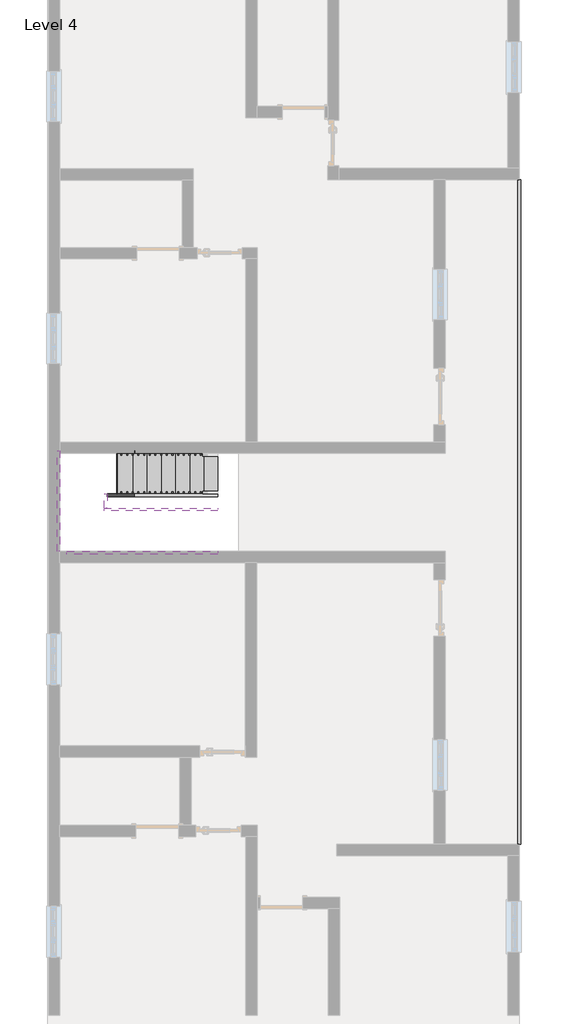
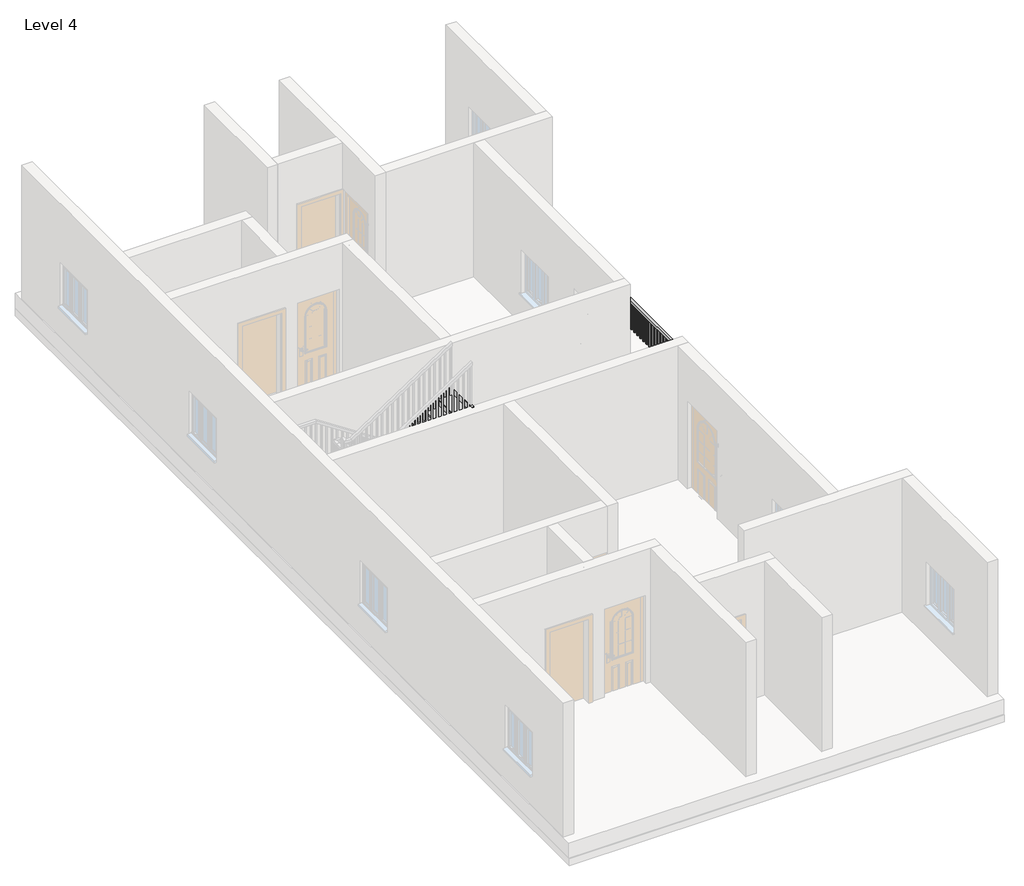
# One storey, part 3 of 3: 6 members, 1 railing, 1 stair flight.
"""IFC4 building model written with IfcOpenShell, lengths in millimetres."""

from ifc_helpers import new_model, si_unit, frame, origin, place, context, project, spatial, polyline, outline, extrude, transform, mapped, element, save
from components import stair_flight_94c6aef5

model = new_model("IFC4")

# Units and contexts
model_context = context("Model", 3, world=origin())
ifc_project = project(units=[si_unit("LENGTHUNIT", "METRE", prefix="MILLI")], contexts=[model_context])

# Site, building, storey
site = spatial("IfcSite", under=ifc_project)
building = spatial("IfcBuilding", under=site)
storey = spatial("IfcBuildingStorey", under=building, Name="Level 4", Elevation=9144.0)

# Members
placement = place(None, origin())
element("IfcMember", 1, ObjectType="Stringer - 2\" Width", at=placement, inside=storey, context=model_context, shape_type="SweptSolid", body=[
    extrude(outline(polyline([(9144.0, -2118.1728655), (9361.4747739, -2118.1728655), (10671.2681072, -4099.3728655), (10305.8806735, -4099.3728655), (9144.0, -2341.9063005), (9144.0, -2118.1728655)])), frame((0.0, 417.8797121, 0.0), z_axis=(0.0, 1.0, 0.0), x_axis=(0.0, 0.0, 1.0)), (0.0, 0.0, 1.0), 50.8),
])
element("IfcMember", 2, ObjectType="Stringer - 2\" Width", at=placement, inside=storey, context=model_context, shape_type="SweptSolid", body=[
    extrude(outline(polyline([(-4150.1728655, 468.6797121), (-4099.3728655, 468.6797121), (-4099.3728655, 214.6797121), (-4150.1728655, 214.6797121), (-4150.1728655, 468.6797121)])), frame((0.0, 0.0, 10426.7), z_axis=(0.0, 0.0, 1.0), x_axis=(1.0, 0.0, 0.0)), (0.0, 0.0, 1.0), 304.8),
])
element("IfcMember", 3, ObjectType="Stringer - 2\" Width", at=placement, inside=storey, context=model_context, shape_type="SweptSolid", body=[
    extrude(outline(polyline([(10872.7747739, -4150.1728655), (10507.3873402, -4150.1728655), (11850.765118, -2118.1728655), (12216.1525517, -2118.1728655), (10872.7747739, -4150.1728655)])), frame((0.0, 163.8797121, 0.0), z_axis=(0.0, 1.0, 0.0), x_axis=(0.0, 0.0, 1.0)), (0.0, 0.0, 1.0), 50.8),
])
element("IfcMember", 4, ObjectType="Stringer - 2\" Width", at=placement, inside=storey, context=model_context, shape_type="SweptSolid", body=[
    extrude(outline(polyline([(9144.0, -2118.1728655), (9361.4747739, -2118.1728655), (10731.5, -4190.4799301), (10731.5, -4743.1668047), (9144.0, -2341.9063005), (9144.0, -2118.1728655)])), frame((0.0, 1192.5797121, 0.0), z_axis=(0.0, 1.0, 0.0), x_axis=(0.0, 0.0, 1.0)), (0.0, 0.0, 1.0), 50.8),
])
element("IfcMember", 5, ObjectType="Stringer - 2\" Width", at=placement, inside=storey, context=model_context, shape_type="SweptSolid", body=[
    extrude(outline(polyline([(-4994.7394105, 1243.3797121), (-4943.9394105, 1243.3797121), (-4943.9394105, -560.0202879), (-4994.7394105, -560.0202879), (-4994.7394105, 1243.3797121)])), frame((0.0, 0.0, 10426.7), z_axis=(0.0, 0.0, 1.0), x_axis=(1.0, 0.0, 0.0)), (0.0, 0.0, 1.0), 304.8),
])
element("IfcMember", 6, ObjectType="Stringer - 2\" Width", at=placement, inside=storey, context=model_context, shape_type="SweptSolid", body=[
    extrude(outline(polyline([(10426.7, -4272.2209431), (11850.765118, -2118.1728655), (12216.1525517, -2118.1728655), (10426.7, -4824.9078176), (10426.7, -4272.2209431)])), frame((0.0, -610.8202879, 0.0), z_axis=(0.0, 1.0, 0.0), x_axis=(0.0, 0.0, 1.0)), (0.0, 0.0, 1.0), 50.8),
])

# Railing
element("IfcRailing", 7, ObjectType="Handrail - Rectangular", at=placement, inside=storey, context=model_context, shape_type="SweptSolid", body=[
    extrude(outline(polyline([(3298.3605895, -5805.1202879), (3247.5605895, -5805.1202879), (3247.5605895, 6094.2483916), (3298.3605895, 6094.2483916), (3298.3605895, -5805.1202879)])), frame((0.0, 0.0, 10007.6), z_axis=(0.0, 0.0, 1.0), x_axis=(1.0, 0.0, 0.0)), (0.0, 0.0, 1.0), 50.8),
    extrude(outline(polyline([(3282.4855895, 6072.5547121), (3263.4355895, 6072.5547121), (3263.4355895, 6091.6047121), (3282.4855895, 6091.6047121), (3282.4855895, 6072.5547121)])), frame((0.0, 0.0, 9144.0), z_axis=(0.0, 0.0, 1.0), x_axis=(1.0, 0.0, 0.0)), (0.0, 0.0, 1.0), 863.6),
    extrude(outline(polyline([(3282.4855895, 5970.9547121), (3263.4355895, 5970.9547121), (3263.4355895, 5990.0047121), (3282.4855895, 5990.0047121), (3282.4855895, 5970.9547121)])), frame((0.0, 0.0, 9144.0), z_axis=(0.0, 0.0, 1.0), x_axis=(1.0, 0.0, 0.0)), (0.0, 0.0, 1.0), 863.6),
    extrude(outline(polyline([(3282.4855895, 5869.3547121), (3263.4355895, 5869.3547121), (3263.4355895, 5888.4047121), (3282.4855895, 5888.4047121), (3282.4855895, 5869.3547121)])), frame((0.0, 0.0, 9144.0), z_axis=(0.0, 0.0, 1.0), x_axis=(1.0, 0.0, 0.0)), (0.0, 0.0, 1.0), 863.6),
    extrude(outline(polyline([(3282.4855895, 5767.7547121), (3263.4355895, 5767.7547121), (3263.4355895, 5786.8047121), (3282.4855895, 5786.8047121), (3282.4855895, 5767.7547121)])), frame((0.0, 0.0, 9144.0), z_axis=(0.0, 0.0, 1.0), x_axis=(1.0, 0.0, 0.0)), (0.0, 0.0, 1.0), 863.6),
    extrude(outline(polyline([(3282.4855895, 5666.1547121), (3263.4355895, 5666.1547121), (3263.4355895, 5685.2047121), (3282.4855895, 5685.2047121), (3282.4855895, 5666.1547121)])), frame((0.0, 0.0, 9144.0), z_axis=(0.0, 0.0, 1.0), x_axis=(1.0, 0.0, 0.0)), (0.0, 0.0, 1.0), 863.6),
    extrude(outline(polyline([(3282.4855895, 5564.5547121), (3263.4355895, 5564.5547121), (3263.4355895, 5583.6047121), (3282.4855895, 5583.6047121), (3282.4855895, 5564.5547121)])), frame((0.0, 0.0, 9144.0), z_axis=(0.0, 0.0, 1.0), x_axis=(1.0, 0.0, 0.0)), (0.0, 0.0, 1.0), 863.6),
    extrude(outline(polyline([(3282.4855895, 5462.9547121), (3263.4355895, 5462.9547121), (3263.4355895, 5482.0047121), (3282.4855895, 5482.0047121), (3282.4855895, 5462.9547121)])), frame((0.0, 0.0, 9144.0), z_axis=(0.0, 0.0, 1.0), x_axis=(1.0, 0.0, 0.0)), (0.0, 0.0, 1.0), 863.6),
    extrude(outline(polyline([(3282.4855895, 5361.3547121), (3263.4355895, 5361.3547121), (3263.4355895, 5380.4047121), (3282.4855895, 5380.4047121), (3282.4855895, 5361.3547121)])), frame((0.0, 0.0, 9144.0), z_axis=(0.0, 0.0, 1.0), x_axis=(1.0, 0.0, 0.0)), (0.0, 0.0, 1.0), 863.6),
    extrude(outline(polyline([(3282.4855895, 5259.7547121), (3263.4355895, 5259.7547121), (3263.4355895, 5278.8047121), (3282.4855895, 5278.8047121), (3282.4855895, 5259.7547121)])), frame((0.0, 0.0, 9144.0), z_axis=(0.0, 0.0, 1.0), x_axis=(1.0, 0.0, 0.0)), (0.0, 0.0, 1.0), 863.6),
    extrude(outline(polyline([(3282.4855895, 5158.1547121), (3263.4355895, 5158.1547121), (3263.4355895, 5177.2047121), (3282.4855895, 5177.2047121), (3282.4855895, 5158.1547121)])), frame((0.0, 0.0, 9144.0), z_axis=(0.0, 0.0, 1.0), x_axis=(1.0, 0.0, 0.0)), (0.0, 0.0, 1.0), 863.6),
    extrude(outline(polyline([(3282.4855895, 5056.5547121), (3263.4355895, 5056.5547121), (3263.4355895, 5075.6047121), (3282.4855895, 5075.6047121), (3282.4855895, 5056.5547121)])), frame((0.0, 0.0, 9144.0), z_axis=(0.0, 0.0, 1.0), x_axis=(1.0, 0.0, 0.0)), (0.0, 0.0, 1.0), 863.6),
    extrude(outline(polyline([(3282.4855895, 4954.9547121), (3263.4355895, 4954.9547121), (3263.4355895, 4974.0047121), (3282.4855895, 4974.0047121), (3282.4855895, 4954.9547121)])), frame((0.0, 0.0, 9144.0), z_axis=(0.0, 0.0, 1.0), x_axis=(1.0, 0.0, 0.0)), (0.0, 0.0, 1.0), 863.6),
    extrude(outline(polyline([(3282.4855895, 4853.3547121), (3263.4355895, 4853.3547121), (3263.4355895, 4872.4047121), (3282.4855895, 4872.4047121), (3282.4855895, 4853.3547121)])), frame((0.0, 0.0, 9144.0), z_axis=(0.0, 0.0, 1.0), x_axis=(1.0, 0.0, 0.0)), (0.0, 0.0, 1.0), 863.6),
    extrude(outline(polyline([(3282.4855895, 4751.7547121), (3263.4355895, 4751.7547121), (3263.4355895, 4770.8047121), (3282.4855895, 4770.8047121), (3282.4855895, 4751.7547121)])), frame((0.0, 0.0, 9144.0), z_axis=(0.0, 0.0, 1.0), x_axis=(1.0, 0.0, 0.0)), (0.0, 0.0, 1.0), 863.6),
    extrude(outline(polyline([(3282.4855895, 4650.1547121), (3263.4355895, 4650.1547121), (3263.4355895, 4669.2047121), (3282.4855895, 4669.2047121), (3282.4855895, 4650.1547121)])), frame((0.0, 0.0, 9144.0), z_axis=(0.0, 0.0, 1.0), x_axis=(1.0, 0.0, 0.0)), (0.0, 0.0, 1.0), 863.6),
    extrude(outline(polyline([(3282.4855895, 4548.5547121), (3263.4355895, 4548.5547121), (3263.4355895, 4567.6047121), (3282.4855895, 4567.6047121), (3282.4855895, 4548.5547121)])), frame((0.0, 0.0, 9144.0), z_axis=(0.0, 0.0, 1.0), x_axis=(1.0, 0.0, 0.0)), (0.0, 0.0, 1.0), 863.6),
    extrude(outline(polyline([(3282.4855895, 4446.9547121), (3263.4355895, 4446.9547121), (3263.4355895, 4466.0047121), (3282.4855895, 4466.0047121), (3282.4855895, 4446.9547121)])), frame((0.0, 0.0, 9144.0), z_axis=(0.0, 0.0, 1.0), x_axis=(1.0, 0.0, 0.0)), (0.0, 0.0, 1.0), 863.6),
    extrude(outline(polyline([(3282.4855895, 4345.3547121), (3263.4355895, 4345.3547121), (3263.4355895, 4364.4047121), (3282.4855895, 4364.4047121), (3282.4855895, 4345.3547121)])), frame((0.0, 0.0, 9144.0), z_axis=(0.0, 0.0, 1.0), x_axis=(1.0, 0.0, 0.0)), (0.0, 0.0, 1.0), 863.6),
    extrude(outline(polyline([(3282.4855895, 4243.7547121), (3263.4355895, 4243.7547121), (3263.4355895, 4262.8047121), (3282.4855895, 4262.8047121), (3282.4855895, 4243.7547121)])), frame((0.0, 0.0, 9144.0), z_axis=(0.0, 0.0, 1.0), x_axis=(1.0, 0.0, 0.0)), (0.0, 0.0, 1.0), 863.6),
    extrude(outline(polyline([(3282.4855895, 4142.1547121), (3263.4355895, 4142.1547121), (3263.4355895, 4161.2047121), (3282.4855895, 4161.2047121), (3282.4855895, 4142.1547121)])), frame((0.0, 0.0, 9144.0), z_axis=(0.0, 0.0, 1.0), x_axis=(1.0, 0.0, 0.0)), (0.0, 0.0, 1.0), 863.6),
    extrude(outline(polyline([(3282.4855895, 4040.5547121), (3263.4355895, 4040.5547121), (3263.4355895, 4059.6047121), (3282.4855895, 4059.6047121), (3282.4855895, 4040.5547121)])), frame((0.0, 0.0, 9144.0), z_axis=(0.0, 0.0, 1.0), x_axis=(1.0, 0.0, 0.0)), (0.0, 0.0, 1.0), 863.6),
    extrude(outline(polyline([(3282.4855895, 3938.9547121), (3263.4355895, 3938.9547121), (3263.4355895, 3958.0047121), (3282.4855895, 3958.0047121), (3282.4855895, 3938.9547121)])), frame((0.0, 0.0, 9144.0), z_axis=(0.0, 0.0, 1.0), x_axis=(1.0, 0.0, 0.0)), (0.0, 0.0, 1.0), 863.6),
    extrude(outline(polyline([(3282.4855895, 3837.3547121), (3263.4355895, 3837.3547121), (3263.4355895, 3856.4047121), (3282.4855895, 3856.4047121), (3282.4855895, 3837.3547121)])), frame((0.0, 0.0, 9144.0), z_axis=(0.0, 0.0, 1.0), x_axis=(1.0, 0.0, 0.0)), (0.0, 0.0, 1.0), 863.6),
    extrude(outline(polyline([(3282.4855895, 3735.7547121), (3263.4355895, 3735.7547121), (3263.4355895, 3754.8047121), (3282.4855895, 3754.8047121), (3282.4855895, 3735.7547121)])), frame((0.0, 0.0, 9144.0), z_axis=(0.0, 0.0, 1.0), x_axis=(1.0, 0.0, 0.0)), (0.0, 0.0, 1.0), 863.6),
    extrude(outline(polyline([(3282.4855895, 3634.1547121), (3263.4355895, 3634.1547121), (3263.4355895, 3653.2047121), (3282.4855895, 3653.2047121), (3282.4855895, 3634.1547121)])), frame((0.0, 0.0, 9144.0), z_axis=(0.0, 0.0, 1.0), x_axis=(1.0, 0.0, 0.0)), (0.0, 0.0, 1.0), 863.6),
    extrude(outline(polyline([(3282.4855895, 3532.5547121), (3263.4355895, 3532.5547121), (3263.4355895, 3551.6047121), (3282.4855895, 3551.6047121), (3282.4855895, 3532.5547121)])), frame((0.0, 0.0, 9144.0), z_axis=(0.0, 0.0, 1.0), x_axis=(1.0, 0.0, 0.0)), (0.0, 0.0, 1.0), 863.6),
    extrude(outline(polyline([(3282.4855895, 3430.9547121), (3263.4355895, 3430.9547121), (3263.4355895, 3450.0047121), (3282.4855895, 3450.0047121), (3282.4855895, 3430.9547121)])), frame((0.0, 0.0, 9144.0), z_axis=(0.0, 0.0, 1.0), x_axis=(1.0, 0.0, 0.0)), (0.0, 0.0, 1.0), 863.6),
    extrude(outline(polyline([(3282.4855895, 3329.3547121), (3263.4355895, 3329.3547121), (3263.4355895, 3348.4047121), (3282.4855895, 3348.4047121), (3282.4855895, 3329.3547121)])), frame((0.0, 0.0, 9144.0), z_axis=(0.0, 0.0, 1.0), x_axis=(1.0, 0.0, 0.0)), (0.0, 0.0, 1.0), 863.6),
    extrude(outline(polyline([(3282.4855895, 3227.7547121), (3263.4355895, 3227.7547121), (3263.4355895, 3246.8047121), (3282.4855895, 3246.8047121), (3282.4855895, 3227.7547121)])), frame((0.0, 0.0, 9144.0), z_axis=(0.0, 0.0, 1.0), x_axis=(1.0, 0.0, 0.0)), (0.0, 0.0, 1.0), 863.6),
    extrude(outline(polyline([(3282.4855895, 3126.1547121), (3263.4355895, 3126.1547121), (3263.4355895, 3145.2047121), (3282.4855895, 3145.2047121), (3282.4855895, 3126.1547121)])), frame((0.0, 0.0, 9144.0), z_axis=(0.0, 0.0, 1.0), x_axis=(1.0, 0.0, 0.0)), (0.0, 0.0, 1.0), 863.6),
    extrude(outline(polyline([(3282.4855895, 3024.5547121), (3263.4355895, 3024.5547121), (3263.4355895, 3043.6047121), (3282.4855895, 3043.6047121), (3282.4855895, 3024.5547121)])), frame((0.0, 0.0, 9144.0), z_axis=(0.0, 0.0, 1.0), x_axis=(1.0, 0.0, 0.0)), (0.0, 0.0, 1.0), 863.6),
    extrude(outline(polyline([(3282.4855895, 2922.9547121), (3263.4355895, 2922.9547121), (3263.4355895, 2942.0047121), (3282.4855895, 2942.0047121), (3282.4855895, 2922.9547121)])), frame((0.0, 0.0, 9144.0), z_axis=(0.0, 0.0, 1.0), x_axis=(1.0, 0.0, 0.0)), (0.0, 0.0, 1.0), 863.6),
    extrude(outline(polyline([(3282.4855895, 2821.3547121), (3263.4355895, 2821.3547121), (3263.4355895, 2840.4047121), (3282.4855895, 2840.4047121), (3282.4855895, 2821.3547121)])), frame((0.0, 0.0, 9144.0), z_axis=(0.0, 0.0, 1.0), x_axis=(1.0, 0.0, 0.0)), (0.0, 0.0, 1.0), 863.6),
    extrude(outline(polyline([(3282.4855895, 2719.7547121), (3263.4355895, 2719.7547121), (3263.4355895, 2738.8047121), (3282.4855895, 2738.8047121), (3282.4855895, 2719.7547121)])), frame((0.0, 0.0, 9144.0), z_axis=(0.0, 0.0, 1.0), x_axis=(1.0, 0.0, 0.0)), (0.0, 0.0, 1.0), 863.6),
    extrude(outline(polyline([(3282.4855895, 2618.1547121), (3263.4355895, 2618.1547121), (3263.4355895, 2637.2047121), (3282.4855895, 2637.2047121), (3282.4855895, 2618.1547121)])), frame((0.0, 0.0, 9144.0), z_axis=(0.0, 0.0, 1.0), x_axis=(1.0, 0.0, 0.0)), (0.0, 0.0, 1.0), 863.6),
    extrude(outline(polyline([(3282.4855895, 2516.5547121), (3263.4355895, 2516.5547121), (3263.4355895, 2535.6047121), (3282.4855895, 2535.6047121), (3282.4855895, 2516.5547121)])), frame((0.0, 0.0, 9144.0), z_axis=(0.0, 0.0, 1.0), x_axis=(1.0, 0.0, 0.0)), (0.0, 0.0, 1.0), 863.6),
    extrude(outline(polyline([(3282.4855895, 2414.9547121), (3263.4355895, 2414.9547121), (3263.4355895, 2434.0047121), (3282.4855895, 2434.0047121), (3282.4855895, 2414.9547121)])), frame((0.0, 0.0, 9144.0), z_axis=(0.0, 0.0, 1.0), x_axis=(1.0, 0.0, 0.0)), (0.0, 0.0, 1.0), 863.6),
    extrude(outline(polyline([(3282.4855895, 2313.3547121), (3263.4355895, 2313.3547121), (3263.4355895, 2332.4047121), (3282.4855895, 2332.4047121), (3282.4855895, 2313.3547121)])), frame((0.0, 0.0, 9144.0), z_axis=(0.0, 0.0, 1.0), x_axis=(1.0, 0.0, 0.0)), (0.0, 0.0, 1.0), 863.6),
    extrude(outline(polyline([(3282.4855895, 2211.7547121), (3263.4355895, 2211.7547121), (3263.4355895, 2230.8047121), (3282.4855895, 2230.8047121), (3282.4855895, 2211.7547121)])), frame((0.0, 0.0, 9144.0), z_axis=(0.0, 0.0, 1.0), x_axis=(1.0, 0.0, 0.0)), (0.0, 0.0, 1.0), 863.6),
    extrude(outline(polyline([(3282.4855895, 2110.1547121), (3263.4355895, 2110.1547121), (3263.4355895, 2129.2047121), (3282.4855895, 2129.2047121), (3282.4855895, 2110.1547121)])), frame((0.0, 0.0, 9144.0), z_axis=(0.0, 0.0, 1.0), x_axis=(1.0, 0.0, 0.0)), (0.0, 0.0, 1.0), 863.6),
    extrude(outline(polyline([(3282.4855895, 2008.5547121), (3263.4355895, 2008.5547121), (3263.4355895, 2027.6047121), (3282.4855895, 2027.6047121), (3282.4855895, 2008.5547121)])), frame((0.0, 0.0, 9144.0), z_axis=(0.0, 0.0, 1.0), x_axis=(1.0, 0.0, 0.0)), (0.0, 0.0, 1.0), 863.6),
    extrude(outline(polyline([(3282.4855895, 1906.9547121), (3263.4355895, 1906.9547121), (3263.4355895, 1926.0047121), (3282.4855895, 1926.0047121), (3282.4855895, 1906.9547121)])), frame((0.0, 0.0, 9144.0), z_axis=(0.0, 0.0, 1.0), x_axis=(1.0, 0.0, 0.0)), (0.0, 0.0, 1.0), 863.6),
    extrude(outline(polyline([(3282.4855895, 1805.3547121), (3263.4355895, 1805.3547121), (3263.4355895, 1824.4047121), (3282.4855895, 1824.4047121), (3282.4855895, 1805.3547121)])), frame((0.0, 0.0, 9144.0), z_axis=(0.0, 0.0, 1.0), x_axis=(1.0, 0.0, 0.0)), (0.0, 0.0, 1.0), 863.6),
    extrude(outline(polyline([(3282.4855895, 1703.7547121), (3263.4355895, 1703.7547121), (3263.4355895, 1722.8047121), (3282.4855895, 1722.8047121), (3282.4855895, 1703.7547121)])), frame((0.0, 0.0, 9144.0), z_axis=(0.0, 0.0, 1.0), x_axis=(1.0, 0.0, 0.0)), (0.0, 0.0, 1.0), 863.6),
    extrude(outline(polyline([(3282.4855895, 1602.1547121), (3263.4355895, 1602.1547121), (3263.4355895, 1621.2047121), (3282.4855895, 1621.2047121), (3282.4855895, 1602.1547121)])), frame((0.0, 0.0, 9144.0), z_axis=(0.0, 0.0, 1.0), x_axis=(1.0, 0.0, 0.0)), (0.0, 0.0, 1.0), 863.6),
    extrude(outline(polyline([(3282.4855895, 1500.5547121), (3263.4355895, 1500.5547121), (3263.4355895, 1519.6047121), (3282.4855895, 1519.6047121), (3282.4855895, 1500.5547121)])), frame((0.0, 0.0, 9144.0), z_axis=(0.0, 0.0, 1.0), x_axis=(1.0, 0.0, 0.0)), (0.0, 0.0, 1.0), 863.6),
    extrude(outline(polyline([(3282.4855895, 1398.9547121), (3263.4355895, 1398.9547121), (3263.4355895, 1418.0047121), (3282.4855895, 1418.0047121), (3282.4855895, 1398.9547121)])), frame((0.0, 0.0, 9144.0), z_axis=(0.0, 0.0, 1.0), x_axis=(1.0, 0.0, 0.0)), (0.0, 0.0, 1.0), 863.6),
    extrude(outline(polyline([(3282.4855895, 1297.3547121), (3263.4355895, 1297.3547121), (3263.4355895, 1316.4047121), (3282.4855895, 1316.4047121), (3282.4855895, 1297.3547121)])), frame((0.0, 0.0, 9144.0), z_axis=(0.0, 0.0, 1.0), x_axis=(1.0, 0.0, 0.0)), (0.0, 0.0, 1.0), 863.6),
    extrude(outline(polyline([(3282.4855895, 1195.7547121), (3263.4355895, 1195.7547121), (3263.4355895, 1214.8047121), (3282.4855895, 1214.8047121), (3282.4855895, 1195.7547121)])), frame((0.0, 0.0, 9144.0), z_axis=(0.0, 0.0, 1.0), x_axis=(1.0, 0.0, 0.0)), (0.0, 0.0, 1.0), 863.6),
    extrude(outline(polyline([(3282.4855895, 1094.1547121), (3263.4355895, 1094.1547121), (3263.4355895, 1113.2047121), (3282.4855895, 1113.2047121), (3282.4855895, 1094.1547121)])), frame((0.0, 0.0, 9144.0), z_axis=(0.0, 0.0, 1.0), x_axis=(1.0, 0.0, 0.0)), (0.0, 0.0, 1.0), 863.6),
    extrude(outline(polyline([(3282.4855895, 992.5547121), (3263.4355895, 992.5547121), (3263.4355895, 1011.6047121), (3282.4855895, 1011.6047121), (3282.4855895, 992.5547121)])), frame((0.0, 0.0, 9144.0), z_axis=(0.0, 0.0, 1.0), x_axis=(1.0, 0.0, 0.0)), (0.0, 0.0, 1.0), 863.6),
    extrude(outline(polyline([(3282.4855895, 890.9547121), (3263.4355895, 890.9547121), (3263.4355895, 910.0047121), (3282.4855895, 910.0047121), (3282.4855895, 890.9547121)])), frame((0.0, 0.0, 9144.0), z_axis=(0.0, 0.0, 1.0), x_axis=(1.0, 0.0, 0.0)), (0.0, 0.0, 1.0), 863.6),
    extrude(outline(polyline([(3282.4855895, 789.3547121), (3263.4355895, 789.3547121), (3263.4355895, 808.4047121), (3282.4855895, 808.4047121), (3282.4855895, 789.3547121)])), frame((0.0, 0.0, 9144.0), z_axis=(0.0, 0.0, 1.0), x_axis=(1.0, 0.0, 0.0)), (0.0, 0.0, 1.0), 863.6),
    extrude(outline(polyline([(3282.4855895, 687.7547121), (3263.4355895, 687.7547121), (3263.4355895, 706.8047121), (3282.4855895, 706.8047121), (3282.4855895, 687.7547121)])), frame((0.0, 0.0, 9144.0), z_axis=(0.0, 0.0, 1.0), x_axis=(1.0, 0.0, 0.0)), (0.0, 0.0, 1.0), 863.6),
    extrude(outline(polyline([(3282.4855895, 586.1547121), (3263.4355895, 586.1547121), (3263.4355895, 605.2047121), (3282.4855895, 605.2047121), (3282.4855895, 586.1547121)])), frame((0.0, 0.0, 9144.0), z_axis=(0.0, 0.0, 1.0), x_axis=(1.0, 0.0, 0.0)), (0.0, 0.0, 1.0), 863.6),
    extrude(outline(polyline([(3282.4855895, 484.5547121), (3263.4355895, 484.5547121), (3263.4355895, 503.6047121), (3282.4855895, 503.6047121), (3282.4855895, 484.5547121)])), frame((0.0, 0.0, 9144.0), z_axis=(0.0, 0.0, 1.0), x_axis=(1.0, 0.0, 0.0)), (0.0, 0.0, 1.0), 863.6),
    extrude(outline(polyline([(3282.4855895, 382.9547121), (3263.4355895, 382.9547121), (3263.4355895, 402.0047121), (3282.4855895, 402.0047121), (3282.4855895, 382.9547121)])), frame((0.0, 0.0, 9144.0), z_axis=(0.0, 0.0, 1.0), x_axis=(1.0, 0.0, 0.0)), (0.0, 0.0, 1.0), 863.6),
    extrude(outline(polyline([(3282.4855895, 281.3547121), (3263.4355895, 281.3547121), (3263.4355895, 300.4047121), (3282.4855895, 300.4047121), (3282.4855895, 281.3547121)])), frame((0.0, 0.0, 9144.0), z_axis=(0.0, 0.0, 1.0), x_axis=(1.0, 0.0, 0.0)), (0.0, 0.0, 1.0), 863.6),
    extrude(outline(polyline([(3282.4855895, 179.7547121), (3263.4355895, 179.7547121), (3263.4355895, 198.8047121), (3282.4855895, 198.8047121), (3282.4855895, 179.7547121)])), frame((0.0, 0.0, 9144.0), z_axis=(0.0, 0.0, 1.0), x_axis=(1.0, 0.0, 0.0)), (0.0, 0.0, 1.0), 863.6),
    extrude(outline(polyline([(3282.4855895, 78.1547121), (3263.4355895, 78.1547121), (3263.4355895, 97.2047121), (3282.4855895, 97.2047121), (3282.4855895, 78.1547121)])), frame((0.0, 0.0, 9144.0), z_axis=(0.0, 0.0, 1.0), x_axis=(1.0, 0.0, 0.0)), (0.0, 0.0, 1.0), 863.6),
    extrude(outline(polyline([(3282.4855895, -23.4452879), (3263.4355895, -23.4452879), (3263.4355895, -4.3952879), (3282.4855895, -4.3952879), (3282.4855895, -23.4452879)])), frame((0.0, 0.0, 9144.0), z_axis=(0.0, 0.0, 1.0), x_axis=(1.0, 0.0, 0.0)), (0.0, 0.0, 1.0), 863.6),
    extrude(outline(polyline([(3282.4855895, -125.0452879), (3263.4355895, -125.0452879), (3263.4355895, -105.9952879), (3282.4855895, -105.9952879), (3282.4855895, -125.0452879)])), frame((0.0, 0.0, 9144.0), z_axis=(0.0, 0.0, 1.0), x_axis=(1.0, 0.0, 0.0)), (0.0, 0.0, 1.0), 863.6),
    extrude(outline(polyline([(3282.4855895, -226.6452879), (3263.4355895, -226.6452879), (3263.4355895, -207.5952879), (3282.4855895, -207.5952879), (3282.4855895, -226.6452879)])), frame((0.0, 0.0, 9144.0), z_axis=(0.0, 0.0, 1.0), x_axis=(1.0, 0.0, 0.0)), (0.0, 0.0, 1.0), 863.6),
    extrude(outline(polyline([(3282.4855895, -328.2452879), (3263.4355895, -328.2452879), (3263.4355895, -309.1952879), (3282.4855895, -309.1952879), (3282.4855895, -328.2452879)])), frame((0.0, 0.0, 9144.0), z_axis=(0.0, 0.0, 1.0), x_axis=(1.0, 0.0, 0.0)), (0.0, 0.0, 1.0), 863.6),
    extrude(outline(polyline([(3282.4855895, -429.8452879), (3263.4355895, -429.8452879), (3263.4355895, -410.7952879), (3282.4855895, -410.7952879), (3282.4855895, -429.8452879)])), frame((0.0, 0.0, 9144.0), z_axis=(0.0, 0.0, 1.0), x_axis=(1.0, 0.0, 0.0)), (0.0, 0.0, 1.0), 863.6),
    extrude(outline(polyline([(3282.4855895, -531.4452879), (3263.4355895, -531.4452879), (3263.4355895, -512.3952879), (3282.4855895, -512.3952879), (3282.4855895, -531.4452879)])), frame((0.0, 0.0, 9144.0), z_axis=(0.0, 0.0, 1.0), x_axis=(1.0, 0.0, 0.0)), (0.0, 0.0, 1.0), 863.6),
    extrude(outline(polyline([(3282.4855895, -633.0452879), (3263.4355895, -633.0452879), (3263.4355895, -613.9952879), (3282.4855895, -613.9952879), (3282.4855895, -633.0452879)])), frame((0.0, 0.0, 9144.0), z_axis=(0.0, 0.0, 1.0), x_axis=(1.0, 0.0, 0.0)), (0.0, 0.0, 1.0), 863.6),
    extrude(outline(polyline([(3282.4855895, -734.6452879), (3263.4355895, -734.6452879), (3263.4355895, -715.5952879), (3282.4855895, -715.5952879), (3282.4855895, -734.6452879)])), frame((0.0, 0.0, 9144.0), z_axis=(0.0, 0.0, 1.0), x_axis=(1.0, 0.0, 0.0)), (0.0, 0.0, 1.0), 863.6),
    extrude(outline(polyline([(3282.4855895, -836.2452879), (3263.4355895, -836.2452879), (3263.4355895, -817.1952879), (3282.4855895, -817.1952879), (3282.4855895, -836.2452879)])), frame((0.0, 0.0, 9144.0), z_axis=(0.0, 0.0, 1.0), x_axis=(1.0, 0.0, 0.0)), (0.0, 0.0, 1.0), 863.6),
    extrude(outline(polyline([(3282.4855895, -937.8452879), (3263.4355895, -937.8452879), (3263.4355895, -918.7952879), (3282.4855895, -918.7952879), (3282.4855895, -937.8452879)])), frame((0.0, 0.0, 9144.0), z_axis=(0.0, 0.0, 1.0), x_axis=(1.0, 0.0, 0.0)), (0.0, 0.0, 1.0), 863.6),
    extrude(outline(polyline([(3282.4855895, -1039.4452879), (3263.4355895, -1039.4452879), (3263.4355895, -1020.3952879), (3282.4855895, -1020.3952879), (3282.4855895, -1039.4452879)])), frame((0.0, 0.0, 9144.0), z_axis=(0.0, 0.0, 1.0), x_axis=(1.0, 0.0, 0.0)), (0.0, 0.0, 1.0), 863.6),
    extrude(outline(polyline([(3282.4855895, -1141.0452879), (3263.4355895, -1141.0452879), (3263.4355895, -1121.9952879), (3282.4855895, -1121.9952879), (3282.4855895, -1141.0452879)])), frame((0.0, 0.0, 9144.0), z_axis=(0.0, 0.0, 1.0), x_axis=(1.0, 0.0, 0.0)), (0.0, 0.0, 1.0), 863.6),
    extrude(outline(polyline([(3282.4855895, -1242.6452879), (3263.4355895, -1242.6452879), (3263.4355895, -1223.5952879), (3282.4855895, -1223.5952879), (3282.4855895, -1242.6452879)])), frame((0.0, 0.0, 9144.0), z_axis=(0.0, 0.0, 1.0), x_axis=(1.0, 0.0, 0.0)), (0.0, 0.0, 1.0), 863.6),
    extrude(outline(polyline([(3282.4855895, -1344.2452879), (3263.4355895, -1344.2452879), (3263.4355895, -1325.1952879), (3282.4855895, -1325.1952879), (3282.4855895, -1344.2452879)])), frame((0.0, 0.0, 9144.0), z_axis=(0.0, 0.0, 1.0), x_axis=(1.0, 0.0, 0.0)), (0.0, 0.0, 1.0), 863.6),
    extrude(outline(polyline([(3282.4855895, -1445.8452879), (3263.4355895, -1445.8452879), (3263.4355895, -1426.7952879), (3282.4855895, -1426.7952879), (3282.4855895, -1445.8452879)])), frame((0.0, 0.0, 9144.0), z_axis=(0.0, 0.0, 1.0), x_axis=(1.0, 0.0, 0.0)), (0.0, 0.0, 1.0), 863.6),
    extrude(outline(polyline([(3282.4855895, -1547.4452879), (3263.4355895, -1547.4452879), (3263.4355895, -1528.3952879), (3282.4855895, -1528.3952879), (3282.4855895, -1547.4452879)])), frame((0.0, 0.0, 9144.0), z_axis=(0.0, 0.0, 1.0), x_axis=(1.0, 0.0, 0.0)), (0.0, 0.0, 1.0), 863.6),
    extrude(outline(polyline([(3282.4855895, -1649.0452879), (3263.4355895, -1649.0452879), (3263.4355895, -1629.9952879), (3282.4855895, -1629.9952879), (3282.4855895, -1649.0452879)])), frame((0.0, 0.0, 9144.0), z_axis=(0.0, 0.0, 1.0), x_axis=(1.0, 0.0, 0.0)), (0.0, 0.0, 1.0), 863.6),
    extrude(outline(polyline([(3282.4855895, -1750.6452879), (3263.4355895, -1750.6452879), (3263.4355895, -1731.5952879), (3282.4855895, -1731.5952879), (3282.4855895, -1750.6452879)])), frame((0.0, 0.0, 9144.0), z_axis=(0.0, 0.0, 1.0), x_axis=(1.0, 0.0, 0.0)), (0.0, 0.0, 1.0), 863.6),
    extrude(outline(polyline([(3282.4855895, -1852.2452879), (3263.4355895, -1852.2452879), (3263.4355895, -1833.1952879), (3282.4855895, -1833.1952879), (3282.4855895, -1852.2452879)])), frame((0.0, 0.0, 9144.0), z_axis=(0.0, 0.0, 1.0), x_axis=(1.0, 0.0, 0.0)), (0.0, 0.0, 1.0), 863.6),
    extrude(outline(polyline([(3282.4855895, -1953.8452879), (3263.4355895, -1953.8452879), (3263.4355895, -1934.7952879), (3282.4855895, -1934.7952879), (3282.4855895, -1953.8452879)])), frame((0.0, 0.0, 9144.0), z_axis=(0.0, 0.0, 1.0), x_axis=(1.0, 0.0, 0.0)), (0.0, 0.0, 1.0), 863.6),
    extrude(outline(polyline([(3282.4855895, -2055.4452879), (3263.4355895, -2055.4452879), (3263.4355895, -2036.3952879), (3282.4855895, -2036.3952879), (3282.4855895, -2055.4452879)])), frame((0.0, 0.0, 9144.0), z_axis=(0.0, 0.0, 1.0), x_axis=(1.0, 0.0, 0.0)), (0.0, 0.0, 1.0), 863.6),
    extrude(outline(polyline([(3282.4855895, -2157.0452879), (3263.4355895, -2157.0452879), (3263.4355895, -2137.9952879), (3282.4855895, -2137.9952879), (3282.4855895, -2157.0452879)])), frame((0.0, 0.0, 9144.0), z_axis=(0.0, 0.0, 1.0), x_axis=(1.0, 0.0, 0.0)), (0.0, 0.0, 1.0), 863.6),
    extrude(outline(polyline([(3282.4855895, -2258.6452879), (3263.4355895, -2258.6452879), (3263.4355895, -2239.5952879), (3282.4855895, -2239.5952879), (3282.4855895, -2258.6452879)])), frame((0.0, 0.0, 9144.0), z_axis=(0.0, 0.0, 1.0), x_axis=(1.0, 0.0, 0.0)), (0.0, 0.0, 1.0), 863.6),
    extrude(outline(polyline([(3282.4855895, -2360.2452879), (3263.4355895, -2360.2452879), (3263.4355895, -2341.1952879), (3282.4855895, -2341.1952879), (3282.4855895, -2360.2452879)])), frame((0.0, 0.0, 9144.0), z_axis=(0.0, 0.0, 1.0), x_axis=(1.0, 0.0, 0.0)), (0.0, 0.0, 1.0), 863.6),
    extrude(outline(polyline([(3282.4855895, -2461.8452879), (3263.4355895, -2461.8452879), (3263.4355895, -2442.7952879), (3282.4855895, -2442.7952879), (3282.4855895, -2461.8452879)])), frame((0.0, 0.0, 9144.0), z_axis=(0.0, 0.0, 1.0), x_axis=(1.0, 0.0, 0.0)), (0.0, 0.0, 1.0), 863.6),
    extrude(outline(polyline([(3282.4855895, -2563.4452879), (3263.4355895, -2563.4452879), (3263.4355895, -2544.3952879), (3282.4855895, -2544.3952879), (3282.4855895, -2563.4452879)])), frame((0.0, 0.0, 9144.0), z_axis=(0.0, 0.0, 1.0), x_axis=(1.0, 0.0, 0.0)), (0.0, 0.0, 1.0), 863.6),
    extrude(outline(polyline([(3282.4855895, -2665.0452879), (3263.4355895, -2665.0452879), (3263.4355895, -2645.9952879), (3282.4855895, -2645.9952879), (3282.4855895, -2665.0452879)])), frame((0.0, 0.0, 9144.0), z_axis=(0.0, 0.0, 1.0), x_axis=(1.0, 0.0, 0.0)), (0.0, 0.0, 1.0), 863.6),
    extrude(outline(polyline([(3282.4855895, -2766.6452879), (3263.4355895, -2766.6452879), (3263.4355895, -2747.5952879), (3282.4855895, -2747.5952879), (3282.4855895, -2766.6452879)])), frame((0.0, 0.0, 9144.0), z_axis=(0.0, 0.0, 1.0), x_axis=(1.0, 0.0, 0.0)), (0.0, 0.0, 1.0), 863.6),
    extrude(outline(polyline([(3282.4855895, -2868.2452879), (3263.4355895, -2868.2452879), (3263.4355895, -2849.1952879), (3282.4855895, -2849.1952879), (3282.4855895, -2868.2452879)])), frame((0.0, 0.0, 9144.0), z_axis=(0.0, 0.0, 1.0), x_axis=(1.0, 0.0, 0.0)), (0.0, 0.0, 1.0), 863.6),
    extrude(outline(polyline([(3282.4855895, -2969.8452879), (3263.4355895, -2969.8452879), (3263.4355895, -2950.7952879), (3282.4855895, -2950.7952879), (3282.4855895, -2969.8452879)])), frame((0.0, 0.0, 9144.0), z_axis=(0.0, 0.0, 1.0), x_axis=(1.0, 0.0, 0.0)), (0.0, 0.0, 1.0), 863.6),
    extrude(outline(polyline([(3282.4855895, -3071.4452879), (3263.4355895, -3071.4452879), (3263.4355895, -3052.3952879), (3282.4855895, -3052.3952879), (3282.4855895, -3071.4452879)])), frame((0.0, 0.0, 9144.0), z_axis=(0.0, 0.0, 1.0), x_axis=(1.0, 0.0, 0.0)), (0.0, 0.0, 1.0), 863.6),
    extrude(outline(polyline([(3282.4855895, -3173.0452879), (3263.4355895, -3173.0452879), (3263.4355895, -3153.9952879), (3282.4855895, -3153.9952879), (3282.4855895, -3173.0452879)])), frame((0.0, 0.0, 9144.0), z_axis=(0.0, 0.0, 1.0), x_axis=(1.0, 0.0, 0.0)), (0.0, 0.0, 1.0), 863.6),
    extrude(outline(polyline([(3282.4855895, -3274.6452879), (3263.4355895, -3274.6452879), (3263.4355895, -3255.5952879), (3282.4855895, -3255.5952879), (3282.4855895, -3274.6452879)])), frame((0.0, 0.0, 9144.0), z_axis=(0.0, 0.0, 1.0), x_axis=(1.0, 0.0, 0.0)), (0.0, 0.0, 1.0), 863.6),
    extrude(outline(polyline([(3282.4855895, -3376.2452879), (3263.4355895, -3376.2452879), (3263.4355895, -3357.1952879), (3282.4855895, -3357.1952879), (3282.4855895, -3376.2452879)])), frame((0.0, 0.0, 9144.0), z_axis=(0.0, 0.0, 1.0), x_axis=(1.0, 0.0, 0.0)), (0.0, 0.0, 1.0), 863.6),
    extrude(outline(polyline([(3282.4855895, -3477.8452879), (3263.4355895, -3477.8452879), (3263.4355895, -3458.7952879), (3282.4855895, -3458.7952879), (3282.4855895, -3477.8452879)])), frame((0.0, 0.0, 9144.0), z_axis=(0.0, 0.0, 1.0), x_axis=(1.0, 0.0, 0.0)), (0.0, 0.0, 1.0), 863.6),
    extrude(outline(polyline([(3282.4855895, -3579.4452879), (3263.4355895, -3579.4452879), (3263.4355895, -3560.3952879), (3282.4855895, -3560.3952879), (3282.4855895, -3579.4452879)])), frame((0.0, 0.0, 9144.0), z_axis=(0.0, 0.0, 1.0), x_axis=(1.0, 0.0, 0.0)), (0.0, 0.0, 1.0), 863.6),
    extrude(outline(polyline([(3282.4855895, -3681.0452879), (3263.4355895, -3681.0452879), (3263.4355895, -3661.9952879), (3282.4855895, -3661.9952879), (3282.4855895, -3681.0452879)])), frame((0.0, 0.0, 9144.0), z_axis=(0.0, 0.0, 1.0), x_axis=(1.0, 0.0, 0.0)), (0.0, 0.0, 1.0), 863.6),
    extrude(outline(polyline([(3282.4855895, -3782.6452879), (3263.4355895, -3782.6452879), (3263.4355895, -3763.5952879), (3282.4855895, -3763.5952879), (3282.4855895, -3782.6452879)])), frame((0.0, 0.0, 9144.0), z_axis=(0.0, 0.0, 1.0), x_axis=(1.0, 0.0, 0.0)), (0.0, 0.0, 1.0), 863.6),
    extrude(outline(polyline([(3282.4855895, -3884.2452879), (3263.4355895, -3884.2452879), (3263.4355895, -3865.1952879), (3282.4855895, -3865.1952879), (3282.4855895, -3884.2452879)])), frame((0.0, 0.0, 9144.0), z_axis=(0.0, 0.0, 1.0), x_axis=(1.0, 0.0, 0.0)), (0.0, 0.0, 1.0), 863.6),
    extrude(outline(polyline([(3282.4855895, -3985.8452879), (3263.4355895, -3985.8452879), (3263.4355895, -3966.7952879), (3282.4855895, -3966.7952879), (3282.4855895, -3985.8452879)])), frame((0.0, 0.0, 9144.0), z_axis=(0.0, 0.0, 1.0), x_axis=(1.0, 0.0, 0.0)), (0.0, 0.0, 1.0), 863.6),
    extrude(outline(polyline([(3282.4855895, -4087.4452879), (3263.4355895, -4087.4452879), (3263.4355895, -4068.3952879), (3282.4855895, -4068.3952879), (3282.4855895, -4087.4452879)])), frame((0.0, 0.0, 9144.0), z_axis=(0.0, 0.0, 1.0), x_axis=(1.0, 0.0, 0.0)), (0.0, 0.0, 1.0), 863.6),
    extrude(outline(polyline([(3282.4855895, -4189.0452879), (3263.4355895, -4189.0452879), (3263.4355895, -4169.9952879), (3282.4855895, -4169.9952879), (3282.4855895, -4189.0452879)])), frame((0.0, 0.0, 9144.0), z_axis=(0.0, 0.0, 1.0), x_axis=(1.0, 0.0, 0.0)), (0.0, 0.0, 1.0), 863.6),
    extrude(outline(polyline([(3282.4855895, -4290.6452879), (3263.4355895, -4290.6452879), (3263.4355895, -4271.5952879), (3282.4855895, -4271.5952879), (3282.4855895, -4290.6452879)])), frame((0.0, 0.0, 9144.0), z_axis=(0.0, 0.0, 1.0), x_axis=(1.0, 0.0, 0.0)), (0.0, 0.0, 1.0), 863.6),
    extrude(outline(polyline([(3282.4855895, -4392.2452879), (3263.4355895, -4392.2452879), (3263.4355895, -4373.1952879), (3282.4855895, -4373.1952879), (3282.4855895, -4392.2452879)])), frame((0.0, 0.0, 9144.0), z_axis=(0.0, 0.0, 1.0), x_axis=(1.0, 0.0, 0.0)), (0.0, 0.0, 1.0), 863.6),
    extrude(outline(polyline([(3282.4855895, -4493.8452879), (3263.4355895, -4493.8452879), (3263.4355895, -4474.7952879), (3282.4855895, -4474.7952879), (3282.4855895, -4493.8452879)])), frame((0.0, 0.0, 9144.0), z_axis=(0.0, 0.0, 1.0), x_axis=(1.0, 0.0, 0.0)), (0.0, 0.0, 1.0), 863.6),
    extrude(outline(polyline([(3282.4855895, -4595.4452879), (3263.4355895, -4595.4452879), (3263.4355895, -4576.3952879), (3282.4855895, -4576.3952879), (3282.4855895, -4595.4452879)])), frame((0.0, 0.0, 9144.0), z_axis=(0.0, 0.0, 1.0), x_axis=(1.0, 0.0, 0.0)), (0.0, 0.0, 1.0), 863.6),
    extrude(outline(polyline([(3282.4855895, -4697.0452879), (3263.4355895, -4697.0452879), (3263.4355895, -4677.9952879), (3282.4855895, -4677.9952879), (3282.4855895, -4697.0452879)])), frame((0.0, 0.0, 9144.0), z_axis=(0.0, 0.0, 1.0), x_axis=(1.0, 0.0, 0.0)), (0.0, 0.0, 1.0), 863.6),
    extrude(outline(polyline([(3282.4855895, -4798.6452879), (3263.4355895, -4798.6452879), (3263.4355895, -4779.5952879), (3282.4855895, -4779.5952879), (3282.4855895, -4798.6452879)])), frame((0.0, 0.0, 9144.0), z_axis=(0.0, 0.0, 1.0), x_axis=(1.0, 0.0, 0.0)), (0.0, 0.0, 1.0), 863.6),
    extrude(outline(polyline([(3282.4855895, -4900.2452879), (3263.4355895, -4900.2452879), (3263.4355895, -4881.1952879), (3282.4855895, -4881.1952879), (3282.4855895, -4900.2452879)])), frame((0.0, 0.0, 9144.0), z_axis=(0.0, 0.0, 1.0), x_axis=(1.0, 0.0, 0.0)), (0.0, 0.0, 1.0), 863.6),
    extrude(outline(polyline([(3282.4855895, -5001.8452879), (3263.4355895, -5001.8452879), (3263.4355895, -4982.7952879), (3282.4855895, -4982.7952879), (3282.4855895, -5001.8452879)])), frame((0.0, 0.0, 9144.0), z_axis=(0.0, 0.0, 1.0), x_axis=(1.0, 0.0, 0.0)), (0.0, 0.0, 1.0), 863.6),
    extrude(outline(polyline([(3282.4855895, -5103.4452879), (3263.4355895, -5103.4452879), (3263.4355895, -5084.3952879), (3282.4855895, -5084.3952879), (3282.4855895, -5103.4452879)])), frame((0.0, 0.0, 9144.0), z_axis=(0.0, 0.0, 1.0), x_axis=(1.0, 0.0, 0.0)), (0.0, 0.0, 1.0), 863.6),
    extrude(outline(polyline([(3282.4855895, -5205.0452879), (3263.4355895, -5205.0452879), (3263.4355895, -5185.9952879), (3282.4855895, -5185.9952879), (3282.4855895, -5205.0452879)])), frame((0.0, 0.0, 9144.0), z_axis=(0.0, 0.0, 1.0), x_axis=(1.0, 0.0, 0.0)), (0.0, 0.0, 1.0), 863.6),
    extrude(outline(polyline([(3282.4855895, -5306.6452879), (3263.4355895, -5306.6452879), (3263.4355895, -5287.5952879), (3282.4855895, -5287.5952879), (3282.4855895, -5306.6452879)])), frame((0.0, 0.0, 9144.0), z_axis=(0.0, 0.0, 1.0), x_axis=(1.0, 0.0, 0.0)), (0.0, 0.0, 1.0), 863.6),
    extrude(outline(polyline([(3282.4855895, -5408.2452879), (3263.4355895, -5408.2452879), (3263.4355895, -5389.1952879), (3282.4855895, -5389.1952879), (3282.4855895, -5408.2452879)])), frame((0.0, 0.0, 9144.0), z_axis=(0.0, 0.0, 1.0), x_axis=(1.0, 0.0, 0.0)), (0.0, 0.0, 1.0), 863.6),
    extrude(outline(polyline([(3282.4855895, -5509.8452879), (3263.4355895, -5509.8452879), (3263.4355895, -5490.7952879), (3282.4855895, -5490.7952879), (3282.4855895, -5509.8452879)])), frame((0.0, 0.0, 9144.0), z_axis=(0.0, 0.0, 1.0), x_axis=(1.0, 0.0, 0.0)), (0.0, 0.0, 1.0), 863.6),
    extrude(outline(polyline([(3282.4855895, -5611.4452879), (3263.4355895, -5611.4452879), (3263.4355895, -5592.3952879), (3282.4855895, -5592.3952879), (3282.4855895, -5611.4452879)])), frame((0.0, 0.0, 9144.0), z_axis=(0.0, 0.0, 1.0), x_axis=(1.0, 0.0, 0.0)), (0.0, 0.0, 1.0), 863.6),
    extrude(outline(polyline([(3282.4855895, -5713.0452879), (3263.4355895, -5713.0452879), (3263.4355895, -5693.9952879), (3282.4855895, -5693.9952879), (3282.4855895, -5713.0452879)])), frame((0.0, 0.0, 9144.0), z_axis=(0.0, 0.0, 1.0), x_axis=(1.0, 0.0, 0.0)), (0.0, 0.0, 1.0), 863.6),
    extrude(outline(polyline([(3282.4855895, 6075.1983916), (3263.4355895, 6075.1983916), (3263.4355895, 6094.2483916), (3282.4855895, 6094.2483916), (3282.4855895, 6075.1983916)])), frame((0.0, 0.0, 9144.0), z_axis=(0.0, 0.0, 1.0), x_axis=(1.0, 0.0, 0.0)), (0.0, 0.0, 1.0), 863.6),
    extrude(outline(polyline([(3282.4855895, -5805.1202879), (3263.4355895, -5805.1202879), (3263.4355895, -5786.0702879), (3282.4855895, -5786.0702879), (3282.4855895, -5805.1202879)])), frame((0.0, 0.0, 9144.0), z_axis=(0.0, 0.0, 1.0), x_axis=(1.0, 0.0, 0.0)), (0.0, 0.0, 1.0), 863.6),
])

# Stair flight
stair_flight_shape = stair_flight_94c6aef5(model_context)
element("IfcStairFlight", 8, ObjectType="2\" Tread 1\" Nosing 1/4\" Riser", at=placement, inside=storey, context=model_context, shape_type="MappedRepresentation", body=[
    mapped(stair_flight_shape, transform((0.0, 0.0, 0.0), x_axis=(1.0, 0.0, 0.0), y_axis=(0.0, 1.0, 0.0), z_axis=(0.0, 0.0, 1.0))),
])

save(model, "model.ifc")

# Revit data of these elements
# Type "Handrail - Rectangular"
#   Assembly Code = "C2010400"
#   built-in parameter 1008612 = 0.0416667 (stored number, unit not read)
#   built-in parameter 1008611 = 0.0416667 (stored number, unit not read)
#   built-in parameter 1008609 = 0.333333 (stored number, unit not read)
#   built-in parameter 1008604 = 0.166667 (stored number, unit not read)
#   built-in parameter 1008603 = 0.166667 (stored number, unit not read)
#   Railing Height = 914.4 mm
#   built-in parameter 1008630 = 2
#   built-in parameter 1008610 = 2
#   built-in parameter 1008618 = Baluster - Square : 3/4"
# Elements 1, 2, 3, 4, 5, 6 (IfcMember, "Stringer - 2\" Width")
#   Phase Created = New Construction
# Element 7 (IfcRailing, "Handrail - Rectangular")
#   Phase Created = New Construction
# Element 8 (IfcStairFlight, "2\" Tread 1\" Nosing 1/4\" Riser")
#   Phase Created = New Construction
